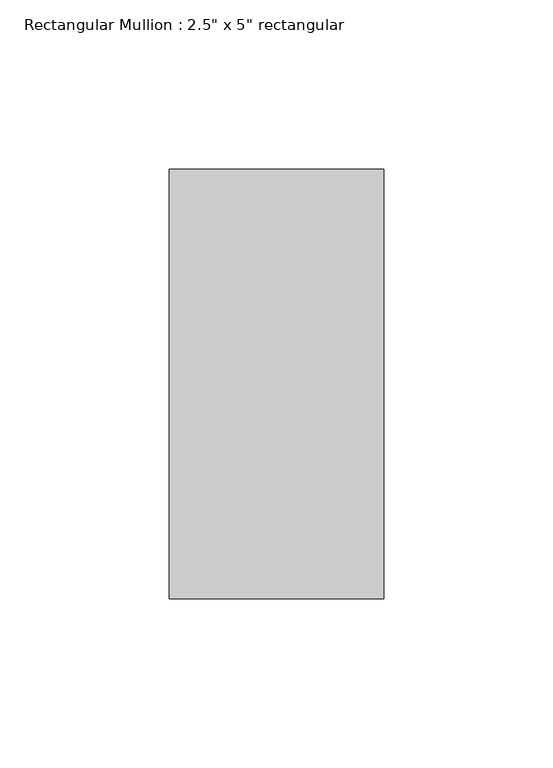
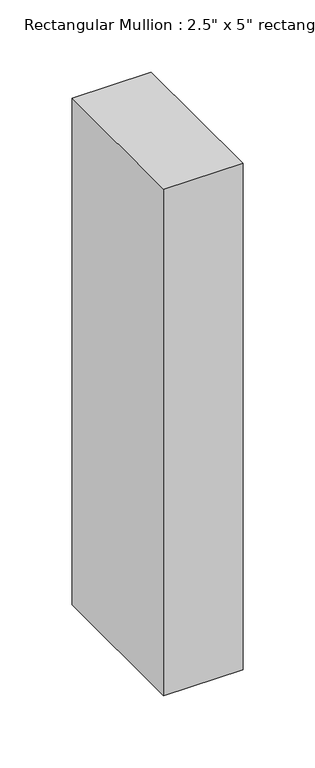
"""IFC4 building model written with IfcOpenShell, lengths in millimetres: member geometry."""

from ifc_helpers import new_model, si_unit, frame, origin, place, context, project, spatial, polyline, outline, extrude, source, transform, mapped, element, save


def member_6b13c281(model_context):
    return source(origin(), model_context, "Body", "SweptSolid", [
        extrude(outline(polyline([(0.0, 63.5), (0.0, -63.5), (-63.5, -63.5), (-63.5, 63.5), (0.0, 63.5)])), frame((0.0, 0.0, -428.625), z_axis=(0.0, 0.0, 1.0), x_axis=(1.0, 0.0, 0.0)), (0.0, 0.0, 1.0), 428.625),
    ])


if __name__ == "__main__":
    model = new_model("IFC4")
    model_context = context("Model", 3, world=origin())
    ifc_project = project(units=[si_unit("LENGTHUNIT", "METRE", prefix="MILLI")], contexts=[model_context])
    site = spatial("IfcSite", under=ifc_project)
    building = spatial("IfcBuilding", under=site)
    placement = place(None, origin())
    member_shape = member_6b13c281(model_context)
    element("IfcMember", 1, ObjectType="Rectangular Mullion : 2.5\" x 5\" rectangular", at=placement, inside=building, context=model_context, shape_type="MappedRepresentation", body=[
        mapped(member_shape, transform((0.0, 0.0, 0.0), x_axis=(1.0, 0.0, 0.0), y_axis=(0.0, 1.0, 0.0), z_axis=(0.0, 0.0, 1.0))),
    ])
    save(model, "model.ifc")

# Revit data of these elements
# Type "Rectangular Mullion : 2.5\" x 5\" rectangular"
#   built-in parameter 1007304 = 0.416667 (stored number, unit not read)
#   built-in parameter 1007301 = 0.104167 (stored number, unit not read)
#   built-in parameter 1007300 = 0.104167 (stored number, unit not read)
# Element 1 (IfcMember, "Rectangular Mullion : 2.5\" x 5\" rectangular")
#   Materials on its faces: "Aluminum"
# Materials
#   "Aluminum": class "Metal", colour RGB 247 247 247, transparency 0, Description = "Aluminum 6061", Cost = 0
